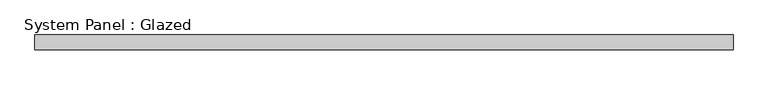
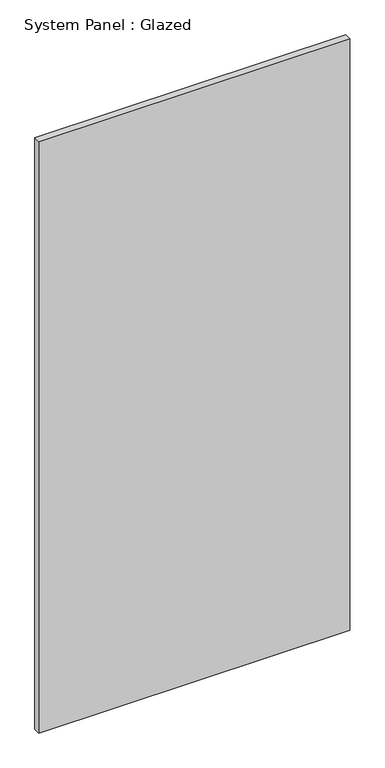
"""IFC4 building model written with IfcOpenShell, lengths in millimetres: plate geometry, System Panel : Glazed."""

from ifc_helpers import new_model, si_unit, origin, origin_with_axes, place, context, project, spatial, polyline, outline, extrude, source, transform, mapped, element, save


def system_panel_glazed_eff01f3a(model_context):
    return source(origin(), model_context, "Body", "SweptSolid", [
        extrude(outline(polyline([(596.6666667, 24.5), (-596.6666667, 24.5), (-596.6666667, 49.5), (596.6666667, 49.5), (596.6666667, 24.5)])), origin_with_axes(), (0.0, 0.0, 1.0), 2400.0),
    ])


if __name__ == "__main__":
    model = new_model("IFC4")
    model_context = context("Model", 3, world=origin())
    ifc_project = project(units=[si_unit("LENGTHUNIT", "METRE", prefix="MILLI")], contexts=[model_context])
    site = spatial("IfcSite", under=ifc_project)
    building = spatial("IfcBuilding", under=site)
    placement = place(None, origin())
    system_panel_glazed_shape = system_panel_glazed_eff01f3a(model_context)
    element("IfcPlate", 1, ObjectType="System Panel : Glazed", at=placement, inside=building, context=model_context, shape_type="MappedRepresentation", body=[
        mapped(system_panel_glazed_shape, transform((0.0, 0.0, 0.0), x_axis=(1.0, 0.0, 0.0), y_axis=(0.0, 1.0, 0.0), z_axis=(0.0, 0.0, 1.0))),
    ])
    save(model, "model.ifc")

# Revit data of these elements
# Type "System Panel : Glazed"
#   Keynote = "H11"
#   Construction Type Id = "GSP4R"
#   Analytic Construction = "1/8 in Pilkington single glazing"
#   Visual Light Transmittance = 0.9
#   Solar Heat Gain Coefficient = 0.86
#   Heat Transfer Coefficient (U) = 6.7069 W/(m²·K)
#   Define Thermal Properties by = 1
# Element 1 (IfcPlate, "System Panel : Glazed")
#   Materials on its faces: "Glass"
# Materials
#   "Glass": class "Glass", colour RGB 0 128 192, transparency 0.9, Description = "Soda Lime Glass", Cost = 0
